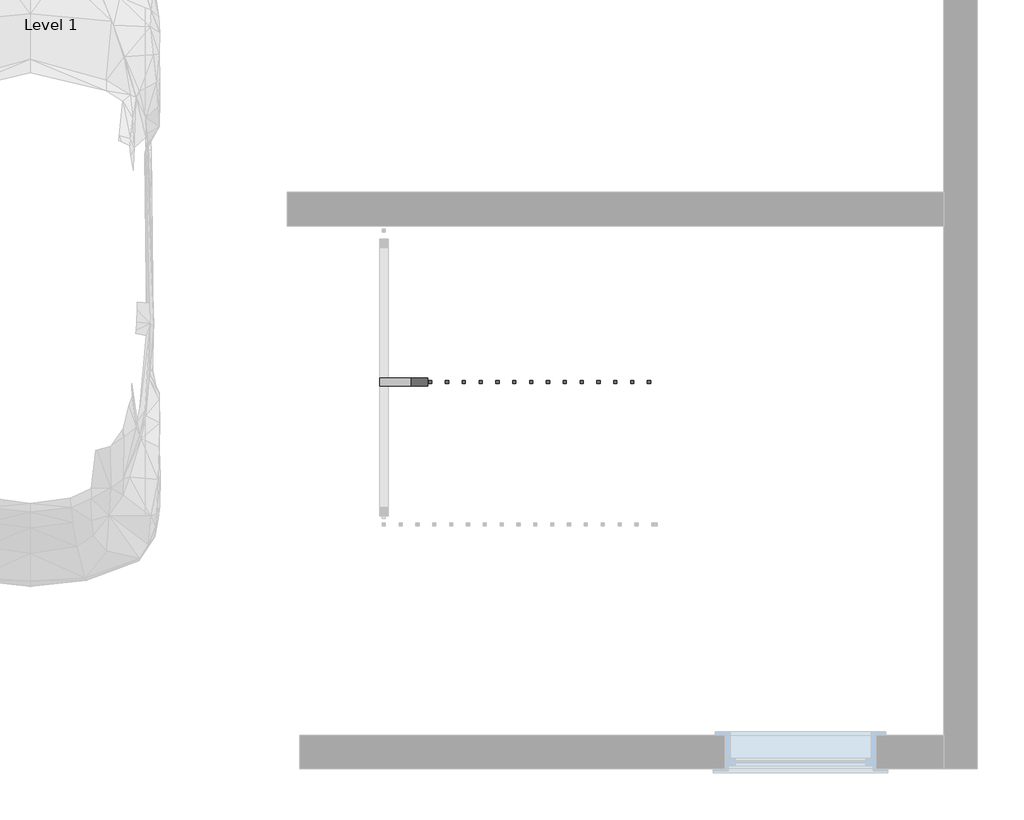
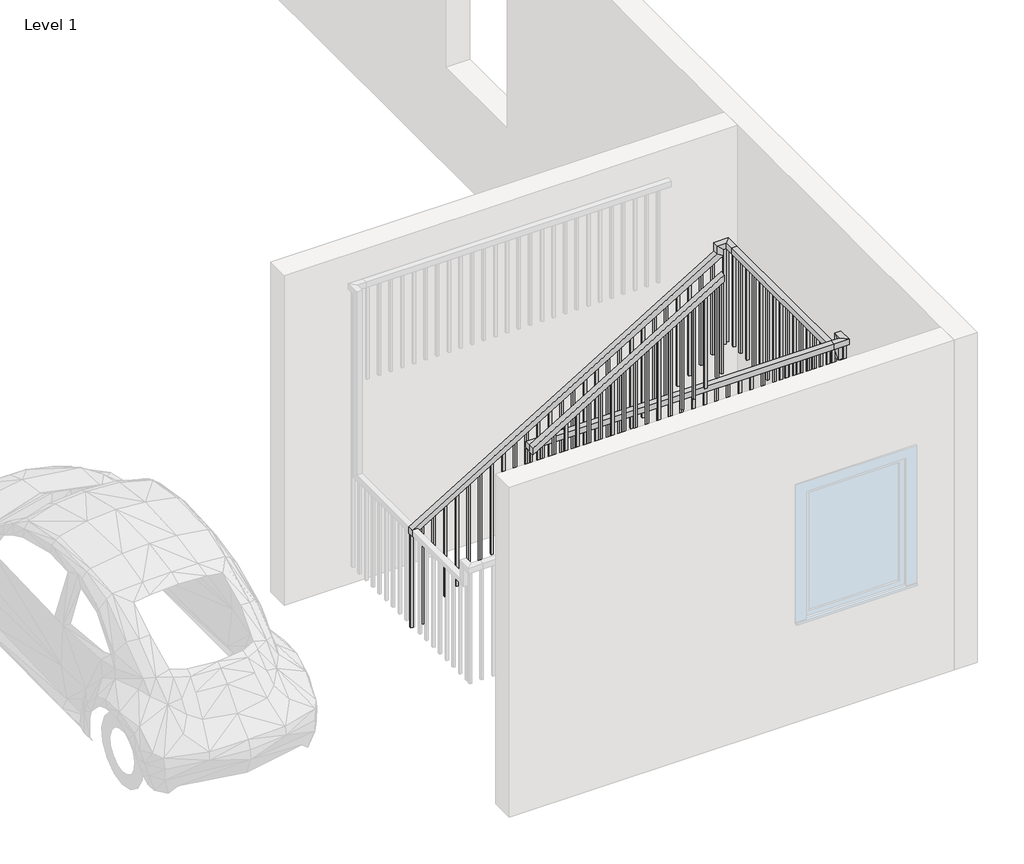
# One storey, part 2 of 3: 1 railing.
"""IFC4 building model written with IfcOpenShell, lengths in millimetres."""

from ifc_helpers import new_model, si_unit, frame, origin, place, context, project, spatial, polyline, outline, extrude, faceted_brep, element, save

model = new_model("IFC4")

# Units and contexts
model_context = context("Model", 3, world=origin())
ifc_project = project(units=[si_unit("LENGTHUNIT", "METRE", prefix="MILLI")], contexts=[model_context])

# Site, building, storey
site = spatial("IfcSite", under=ifc_project)
building = spatial("IfcBuilding", under=site)
storey = spatial("IfcBuildingStorey", under=building, Name="Level 1", Elevation=0.0)

# Railing
placement = place(None, origin())
element("IfcRailing", 1, ObjectType="Handrail - Rectangular", at=placement, inside=storey, context=model_context, shape_type="SolidModel", body=[
    faceted_brep([(-6389.1370113, -4999.3518521, 1083.7333333), (-6389.1370113, -4999.3518521, 1024.3318731), (-6389.1370113, -5050.1518521, 1024.3318731), (-6389.1370113, -5050.1518521, 1083.7333333), (-3722.1370113, -4999.3518521, 2700.0969697), (-3671.3370113, -4999.3518521, 2671.4833882), (-3671.3370113, -5050.1518521, 2671.4833882), (-3722.1370113, -5050.1518521, 2700.0969697), (-3722.1370113, -4999.3518521, 2777.0666667), (-3671.3370113, -4999.3518521, 2726.2666667), (-3671.3370113, -5050.1518521, 2726.2666667), (-3722.1370113, -5050.1518521, 2777.0666667), (-3595.1370113, -4999.3518521, 2777.0666667), (-3595.1370113, -4999.3518521, 2726.2666667), (-3645.9370113, -5050.1518521, 2726.2666667), (-3645.9370113, -5050.1518521, 2777.0666667), (-3595.1370113, -5126.3518521, 2777.0666667), (-3595.1370113, -5126.3518521, 2726.2666667), (-3645.9370113, -5126.3518521, 2726.2666667), (-3645.9370113, -5126.3518521, 2777.0666667), (-3595.1370113, -6697.0215145, 2777.0666667), (-3595.1370113, -6747.8215145, 2726.2666667), (-3645.9370113, -6747.8215145, 2726.2666667), (-3645.9370113, -6697.0215145, 2777.0666667), (-3595.1370113, -6697.0215145, 2946.4), (-3595.1370113, -6747.8215145, 2895.6), (-3645.9370113, -6747.8215145, 2895.6), (-3645.9370113, -6697.0215145, 2946.4), (-3595.1370113, -6824.0215145, 2946.4), (-3595.1370113, -6824.0215145, 2895.6), (-3645.9370113, -6773.2215145, 2895.6), (-3645.9370113, -6773.2215145, 2946.4), (-3722.1370113, -6824.0215145, 2946.4), (-3722.1370113, -6824.0215145, 2895.6), (-3722.1370113, -6773.2215145, 2895.6), (-3722.1370113, -6773.2215145, 2946.4), (-6389.1370113, -6824.0215145, 2946.4), (-6389.1370113, -6773.2215145, 2946.4), (-6389.1370113, -6773.2215145, 2895.6), (-6389.1370113, -6824.0215145, 2895.6)], [[[0, 1, 2, 3]], [[1, 0, 4, 5]], [[2, 1, 5, 6]], [[3, 2, 6, 7]], [[0, 3, 7, 4]], [[5, 4, 8, 9]], [[6, 5, 9, 10]], [[7, 6, 10, 11]], [[4, 7, 11, 8]], [[9, 8, 12, 13]], [[10, 9, 13, 14]], [[11, 10, 14, 15]], [[8, 11, 15, 12]], [[13, 12, 16, 17]], [[14, 13, 17, 18]], [[15, 14, 18, 19]], [[12, 15, 19, 16]], [[17, 16, 20, 21]], [[18, 17, 21, 22]], [[19, 18, 22, 23]], [[16, 19, 23, 20]], [[21, 20, 24, 25]], [[22, 21, 25, 26]], [[23, 22, 26, 27]], [[20, 23, 27, 24]], [[25, 24, 28, 29]], [[26, 25, 29, 30]], [[27, 26, 30, 31]], [[24, 27, 31, 28]], [[29, 28, 32, 33]], [[30, 29, 33, 34]], [[31, 30, 34, 35]], [[28, 31, 35, 32]], [[36, 37, 38, 39]], [[33, 32, 36, 39]], [[34, 33, 39, 38]], [[35, 34, 38, 37]], [[32, 35, 37, 36]]]),
    faceted_brep([(-6389.1370113, -6824.0215145, 2946.4), (-6389.1370113, -6824.0215145, 2886.9985397), (-6389.1370113, -6874.8215145, 2886.9985397), (-6389.1370113, -6874.8215145, 2946.4), (-4712.7370113, -6824.0215145, 3962.4), (-4712.7370113, -6874.8215145, 3962.4), (-4712.7370113, -6874.8215145, 3902.9985397), (-4712.7370113, -6824.0215145, 3902.9985397)], [[[0, 1, 2, 3]], [[4, 5, 6, 7]], [[1, 0, 4, 7]], [[2, 1, 7, 6]], [[3, 2, 6, 5]], [[0, 3, 5, 4]]]),
    extrude(outline(polyline([(3866.4379337, -4773.0620113), (3017.2121212, -4773.0620113), (3017.2121212, -4754.0120113), (3877.9833882, -4754.0120113), (3866.4379337, -4773.0620113)])), frame((0.0, -6858.9465145, 0.0), z_axis=(0.0, 1.0, 0.0), x_axis=(0.0, 0.0, 1.0)), (0.0, 0.0, 1.0), 19.05),
    extrude(outline(polyline([(3804.8621761, -4874.6620113), (2955.6363636, -4874.6620113), (2955.6363636, -4855.6120113), (3816.4076307, -4855.6120113), (3804.8621761, -4874.6620113)])), frame((0.0, -6858.9465145, 0.0), z_axis=(0.0, 1.0, 0.0), x_axis=(0.0, 0.0, 1.0)), (0.0, 0.0, 1.0), 19.05),
    extrude(outline(polyline([(3743.2864185, -4976.2620113), (2894.0606061, -4976.2620113), (2894.0606061, -4957.2120113), (3754.8318731, -4957.2120113), (3743.2864185, -4976.2620113)])), frame((0.0, -6858.9465145, 0.0), z_axis=(0.0, 1.0, 0.0), x_axis=(0.0, 0.0, 1.0)), (0.0, 0.0, 1.0), 19.05),
    extrude(outline(polyline([(3681.710661, -5077.8620113), (2832.4848485, -5077.8620113), (2832.4848485, -5058.8120113), (3693.2561155, -5058.8120113), (3681.710661, -5077.8620113)])), frame((0.0, -6858.9465145, 0.0), z_axis=(0.0, 1.0, 0.0), x_axis=(0.0, 0.0, 1.0)), (0.0, 0.0, 1.0), 19.05),
    extrude(outline(polyline([(3620.1349034, -5179.4620113), (2770.9090909, -5179.4620113), (2770.9090909, -5160.4120113), (3631.6803579, -5160.4120113), (3620.1349034, -5179.4620113)])), frame((0.0, -6858.9465145, 0.0), z_axis=(0.0, 1.0, 0.0), x_axis=(0.0, 0.0, 1.0)), (0.0, 0.0, 1.0), 19.05),
    extrude(outline(polyline([(3558.5591458, -5281.0620113), (2709.3333333, -5281.0620113), (2709.3333333, -5262.0120113), (3570.1046004, -5262.0120113), (3558.5591458, -5281.0620113)])), frame((0.0, -6858.9465145, 0.0), z_axis=(0.0, 1.0, 0.0), x_axis=(0.0, 0.0, 1.0)), (0.0, 0.0, 1.0), 19.05),
    extrude(outline(polyline([(3496.9833882, -5382.6620113), (2647.7575758, -5382.6620113), (2647.7575758, -5363.6120113), (3508.5288428, -5363.6120113), (3496.9833882, -5382.6620113)])), frame((0.0, -6858.9465145, 0.0), z_axis=(0.0, 1.0, 0.0), x_axis=(0.0, 0.0, 1.0)), (0.0, 0.0, 1.0), 19.05),
    extrude(outline(polyline([(3435.4076307, -5484.2620113), (2586.1818182, -5484.2620113), (2586.1818182, -5465.2120113), (3446.9530852, -5465.2120113), (3435.4076307, -5484.2620113)])), frame((0.0, -6858.9465145, 0.0), z_axis=(0.0, 1.0, 0.0), x_axis=(0.0, 0.0, 1.0)), (0.0, 0.0, 1.0), 19.05),
    extrude(outline(polyline([(3373.8318731, -5585.8620113), (2524.6060606, -5585.8620113), (2524.6060606, -5566.8120113), (3385.3773276, -5566.8120113), (3373.8318731, -5585.8620113)])), frame((0.0, -6858.9465145, 0.0), z_axis=(0.0, 1.0, 0.0), x_axis=(0.0, 0.0, 1.0)), (0.0, 0.0, 1.0), 19.05),
    extrude(outline(polyline([(3312.2561155, -5687.4620113), (2463.030303, -5687.4620113), (2463.030303, -5668.4120113), (3323.80157, -5668.4120113), (3312.2561155, -5687.4620113)])), frame((0.0, -6858.9465145, 0.0), z_axis=(0.0, 1.0, 0.0), x_axis=(0.0, 0.0, 1.0)), (0.0, 0.0, 1.0), 19.05),
    extrude(outline(polyline([(3250.6803579, -5789.0620113), (2401.4545455, -5789.0620113), (2401.4545455, -5770.0120113), (3262.2258125, -5770.0120113), (3250.6803579, -5789.0620113)])), frame((0.0, -6858.9465145, 0.0), z_axis=(0.0, 1.0, 0.0), x_axis=(0.0, 0.0, 1.0)), (0.0, 0.0, 1.0), 19.05),
    extrude(outline(polyline([(3189.1046004, -5890.6620113), (2339.8787879, -5890.6620113), (2339.8787879, -5871.6120113), (3200.6500549, -5871.6120113), (3189.1046004, -5890.6620113)])), frame((0.0, -6858.9465145, 0.0), z_axis=(0.0, 1.0, 0.0), x_axis=(0.0, 0.0, 1.0)), (0.0, 0.0, 1.0), 19.05),
    extrude(outline(polyline([(3127.5288428, -5992.2620113), (2278.3030303, -5992.2620113), (2278.3030303, -5973.2120113), (3139.0742973, -5973.2120113), (3127.5288428, -5992.2620113)])), frame((0.0, -6858.9465145, 0.0), z_axis=(0.0, 1.0, 0.0), x_axis=(0.0, 0.0, 1.0)), (0.0, 0.0, 1.0), 19.05),
    extrude(outline(polyline([(3065.9530852, -6093.8620113), (2108.2, -6093.8620113), (2108.2, -6074.8120113), (3077.4985397, -6074.8120113), (3065.9530852, -6093.8620113)])), frame((0.0, -6858.9465145, 0.0), z_axis=(0.0, 1.0, 0.0), x_axis=(0.0, 0.0, 1.0)), (0.0, 0.0, 1.0), 19.05),
    extrude(outline(polyline([(3004.3773276, -6195.4620113), (2108.2, -6195.4620113), (2108.2, -6176.4120113), (3015.9227822, -6176.4120113), (3004.3773276, -6195.4620113)])), frame((0.0, -6858.9465145, 0.0), z_axis=(0.0, 1.0, 0.0), x_axis=(0.0, 0.0, 1.0)), (0.0, 0.0, 1.0), 19.05),
    extrude(outline(polyline([(2942.80157, -6297.0620113), (2108.2, -6297.0620113), (2108.2, -6278.0120113), (2954.3470246, -6278.0120113), (2942.80157, -6297.0620113)])), frame((0.0, -6858.9465145, 0.0), z_axis=(0.0, 1.0, 0.0), x_axis=(0.0, 0.0, 1.0)), (0.0, 0.0, 1.0), 19.05),
    extrude(outline(polyline([(-6354.2120113, -6808.1465145), (-6373.2620113, -6808.1465145), (-6373.2620113, -6789.0965145), (-6354.2120113, -6789.0965145), (-6354.2120113, -6808.1465145)])), frame((0.0, 0.0, 2032.0), z_axis=(0.0, 0.0, 1.0), x_axis=(1.0, 0.0, 0.0)), (0.0, 0.0, 1.0), 863.6),
    extrude(outline(polyline([(2895.6, -6271.6620113), (2157.5236029, -6271.6620113), (2145.9781483, -6252.6120113), (2895.6, -6252.6120113), (2895.6, -6271.6620113)])), frame((0.0, -6808.1465145, 0.0), z_axis=(0.0, 1.0, 0.0), x_axis=(0.0, 0.0, 1.0)), (0.0, 0.0, 1.0), 19.05),
    extrude(outline(polyline([(2895.6, -6170.0620113), (2219.0993604, -6170.0620113), (2207.5539059, -6151.0120113), (2895.6, -6151.0120113), (2895.6, -6170.0620113)])), frame((0.0, -6808.1465145, 0.0), z_axis=(0.0, 1.0, 0.0), x_axis=(0.0, 0.0, 1.0)), (0.0, 0.0, 1.0), 19.05),
    extrude(outline(polyline([(2895.6, -6068.4620113), (2280.675118, -6068.4620113), (2269.1296635, -6049.4120113), (2895.6, -6049.4120113), (2895.6, -6068.4620113)])), frame((0.0, -6808.1465145, 0.0), z_axis=(0.0, 1.0, 0.0), x_axis=(0.0, 0.0, 1.0)), (0.0, 0.0, 1.0), 19.05),
    extrude(outline(polyline([(2895.6, -5966.8620113), (2342.2508756, -5966.8620113), (2330.7054211, -5947.8120113), (2895.6, -5947.8120113), (2895.6, -5966.8620113)])), frame((0.0, -6808.1465145, 0.0), z_axis=(0.0, 1.0, 0.0), x_axis=(0.0, 0.0, 1.0)), (0.0, 0.0, 1.0), 19.05),
    extrude(outline(polyline([(-5846.2120113, -6808.1465145), (-5865.2620113, -6808.1465145), (-5865.2620113, -6789.0965145), (-5846.2120113, -6789.0965145), (-5846.2120113, -6808.1465145)])), frame((0.0, 0.0, 2032.0), z_axis=(0.0, 0.0, 1.0), x_axis=(1.0, 0.0, 0.0)), (0.0, 0.0, 1.0), 863.6),
    extrude(outline(polyline([(-5744.6120113, -6808.1465145), (-5763.6620113, -6808.1465145), (-5763.6620113, -6789.0965145), (-5744.6120113, -6789.0965145), (-5744.6120113, -6808.1465145)])), frame((0.0, 0.0, 2032.0), z_axis=(0.0, 0.0, 1.0), x_axis=(1.0, 0.0, 0.0)), (0.0, 0.0, 1.0), 863.6),
    extrude(outline(polyline([(-5643.0120113, -6808.1465145), (-5662.0620113, -6808.1465145), (-5662.0620113, -6789.0965145), (-5643.0120113, -6789.0965145), (-5643.0120113, -6808.1465145)])), frame((0.0, 0.0, 2032.0), z_axis=(0.0, 0.0, 1.0), x_axis=(1.0, 0.0, 0.0)), (0.0, 0.0, 1.0), 863.6),
    extrude(outline(polyline([(-5541.4120113, -6808.1465145), (-5560.4620113, -6808.1465145), (-5560.4620113, -6789.0965145), (-5541.4120113, -6789.0965145), (-5541.4120113, -6808.1465145)])), frame((0.0, 0.0, 2032.0), z_axis=(0.0, 0.0, 1.0), x_axis=(1.0, 0.0, 0.0)), (0.0, 0.0, 1.0), 863.6),
    extrude(outline(polyline([(-5439.8120113, -6808.1465145), (-5458.8620113, -6808.1465145), (-5458.8620113, -6789.0965145), (-5439.8120113, -6789.0965145), (-5439.8120113, -6808.1465145)])), frame((0.0, 0.0, 2032.0), z_axis=(0.0, 0.0, 1.0), x_axis=(1.0, 0.0, 0.0)), (0.0, 0.0, 1.0), 863.6),
    extrude(outline(polyline([(-5338.2120113, -6808.1465145), (-5357.2620113, -6808.1465145), (-5357.2620113, -6789.0965145), (-5338.2120113, -6789.0965145), (-5338.2120113, -6808.1465145)])), frame((0.0, 0.0, 2032.0), z_axis=(0.0, 0.0, 1.0), x_axis=(1.0, 0.0, 0.0)), (0.0, 0.0, 1.0), 863.6),
    extrude(outline(polyline([(-5236.6120113, -6808.1465145), (-5255.6620113, -6808.1465145), (-5255.6620113, -6789.0965145), (-5236.6120113, -6789.0965145), (-5236.6120113, -6808.1465145)])), frame((0.0, 0.0, 2032.0), z_axis=(0.0, 0.0, 1.0), x_axis=(1.0, 0.0, 0.0)), (0.0, 0.0, 1.0), 863.6),
    extrude(outline(polyline([(-5135.0120113, -6808.1465145), (-5154.0620113, -6808.1465145), (-5154.0620113, -6789.0965145), (-5135.0120113, -6789.0965145), (-5135.0120113, -6808.1465145)])), frame((0.0, 0.0, 2032.0), z_axis=(0.0, 0.0, 1.0), x_axis=(1.0, 0.0, 0.0)), (0.0, 0.0, 1.0), 863.6),
    extrude(outline(polyline([(-5033.4120113, -6808.1465145), (-5052.4620113, -6808.1465145), (-5052.4620113, -6789.0965145), (-5033.4120113, -6789.0965145), (-5033.4120113, -6808.1465145)])), frame((0.0, 0.0, 2032.0), z_axis=(0.0, 0.0, 1.0), x_axis=(1.0, 0.0, 0.0)), (0.0, 0.0, 1.0), 863.6),
    extrude(outline(polyline([(-4931.8120113, -6808.1465145), (-4950.8620113, -6808.1465145), (-4950.8620113, -6789.0965145), (-4931.8120113, -6789.0965145), (-4931.8120113, -6808.1465145)])), frame((0.0, 0.0, 2032.0), z_axis=(0.0, 0.0, 1.0), x_axis=(1.0, 0.0, 0.0)), (0.0, 0.0, 1.0), 863.6),
    extrude(outline(polyline([(-4830.2120113, -6808.1465145), (-4849.2620113, -6808.1465145), (-4849.2620113, -6789.0965145), (-4830.2120113, -6789.0965145), (-4830.2120113, -6808.1465145)])), frame((0.0, 0.0, 2032.0), z_axis=(0.0, 0.0, 1.0), x_axis=(1.0, 0.0, 0.0)), (0.0, 0.0, 1.0), 863.6),
    extrude(outline(polyline([(-4728.6120113, -6808.1465145), (-4747.6620113, -6808.1465145), (-4747.6620113, -6789.0965145), (-4728.6120113, -6789.0965145), (-4728.6120113, -6808.1465145)])), frame((0.0, 0.0, 2032.0), z_axis=(0.0, 0.0, 1.0), x_axis=(1.0, 0.0, 0.0)), (0.0, 0.0, 1.0), 863.6),
    extrude(outline(polyline([(-4627.0120113, -6808.1465145), (-4646.0620113, -6808.1465145), (-4646.0620113, -6789.0965145), (-4627.0120113, -6789.0965145), (-4627.0120113, -6808.1465145)])), frame((0.0, 0.0, 2032.0), z_axis=(0.0, 0.0, 1.0), x_axis=(1.0, 0.0, 0.0)), (0.0, 0.0, 1.0), 863.6),
    extrude(outline(polyline([(-4525.4120113, -6808.1465145), (-4544.4620113, -6808.1465145), (-4544.4620113, -6789.0965145), (-4525.4120113, -6789.0965145), (-4525.4120113, -6808.1465145)])), frame((0.0, 0.0, 2032.0), z_axis=(0.0, 0.0, 1.0), x_axis=(1.0, 0.0, 0.0)), (0.0, 0.0, 1.0), 863.6),
    extrude(outline(polyline([(-4423.8120113, -6808.1465145), (-4442.8620113, -6808.1465145), (-4442.8620113, -6789.0965145), (-4423.8120113, -6789.0965145), (-4423.8120113, -6808.1465145)])), frame((0.0, 0.0, 2032.0), z_axis=(0.0, 0.0, 1.0), x_axis=(1.0, 0.0, 0.0)), (0.0, 0.0, 1.0), 863.6),
    extrude(outline(polyline([(-4322.2120113, -6808.1465145), (-4341.2620113, -6808.1465145), (-4341.2620113, -6789.0965145), (-4322.2120113, -6789.0965145), (-4322.2120113, -6808.1465145)])), frame((0.0, 0.0, 2032.0), z_axis=(0.0, 0.0, 1.0), x_axis=(1.0, 0.0, 0.0)), (0.0, 0.0, 1.0), 863.6),
    extrude(outline(polyline([(-4220.6120113, -6808.1465145), (-4239.6620113, -6808.1465145), (-4239.6620113, -6789.0965145), (-4220.6120113, -6789.0965145), (-4220.6120113, -6808.1465145)])), frame((0.0, 0.0, 2032.0), z_axis=(0.0, 0.0, 1.0), x_axis=(1.0, 0.0, 0.0)), (0.0, 0.0, 1.0), 863.6),
    extrude(outline(polyline([(-4119.0120113, -6808.1465145), (-4138.0620113, -6808.1465145), (-4138.0620113, -6789.0965145), (-4119.0120113, -6789.0965145), (-4119.0120113, -6808.1465145)])), frame((0.0, 0.0, 2032.0), z_axis=(0.0, 0.0, 1.0), x_axis=(1.0, 0.0, 0.0)), (0.0, 0.0, 1.0), 863.6),
    extrude(outline(polyline([(-4017.4120113, -6808.1465145), (-4036.4620113, -6808.1465145), (-4036.4620113, -6789.0965145), (-4017.4120113, -6789.0965145), (-4017.4120113, -6808.1465145)])), frame((0.0, 0.0, 2032.0), z_axis=(0.0, 0.0, 1.0), x_axis=(1.0, 0.0, 0.0)), (0.0, 0.0, 1.0), 863.6),
    extrude(outline(polyline([(-3915.8120113, -6808.1465145), (-3934.8620113, -6808.1465145), (-3934.8620113, -6789.0965145), (-3915.8120113, -6789.0965145), (-3915.8120113, -6808.1465145)])), frame((0.0, 0.0, 2032.0), z_axis=(0.0, 0.0, 1.0), x_axis=(1.0, 0.0, 0.0)), (0.0, 0.0, 1.0), 863.6),
    extrude(outline(polyline([(-3814.2120113, -6808.1465145), (-3833.2620113, -6808.1465145), (-3833.2620113, -6789.0965145), (-3814.2120113, -6789.0965145), (-3814.2120113, -6808.1465145)])), frame((0.0, 0.0, 2032.0), z_axis=(0.0, 0.0, 1.0), x_axis=(1.0, 0.0, 0.0)), (0.0, 0.0, 1.0), 863.6),
    extrude(outline(polyline([(-3712.6120113, -6808.1465145), (-3731.6620113, -6808.1465145), (-3731.6620113, -6789.0965145), (-3712.6120113, -6789.0965145), (-3712.6120113, -6808.1465145)])), frame((0.0, 0.0, 2032.0), z_axis=(0.0, 0.0, 1.0), x_axis=(1.0, 0.0, 0.0)), (0.0, 0.0, 1.0), 863.6),
    extrude(outline(polyline([(-3611.0120113, -6742.4268521), (-3611.0120113, -6761.4768521), (-3630.0620113, -6761.4768521), (-3630.0620113, -6742.4268521), (-3611.0120113, -6742.4268521)])), frame((0.0, 0.0, 1862.6666667), z_axis=(0.0, 0.0, 1.0), x_axis=(1.0, 0.0, 0.0)), (0.0, 0.0, 1.0), 863.6),
    extrude(outline(polyline([(-3611.0120113, -6640.8268521), (-3611.0120113, -6659.8768521), (-3630.0620113, -6659.8768521), (-3630.0620113, -6640.8268521), (-3611.0120113, -6640.8268521)])), frame((0.0, 0.0, 1862.6666667), z_axis=(0.0, 0.0, 1.0), x_axis=(1.0, 0.0, 0.0)), (0.0, 0.0, 1.0), 863.6),
    extrude(outline(polyline([(-3611.0120113, -6539.2268521), (-3611.0120113, -6558.2768521), (-3630.0620113, -6558.2768521), (-3630.0620113, -6539.2268521), (-3611.0120113, -6539.2268521)])), frame((0.0, 0.0, 1862.6666667), z_axis=(0.0, 0.0, 1.0), x_axis=(1.0, 0.0, 0.0)), (0.0, 0.0, 1.0), 863.6),
    extrude(outline(polyline([(-3611.0120113, -6437.6268521), (-3611.0120113, -6456.6768521), (-3630.0620113, -6456.6768521), (-3630.0620113, -6437.6268521), (-3611.0120113, -6437.6268521)])), frame((0.0, 0.0, 1862.6666667), z_axis=(0.0, 0.0, 1.0), x_axis=(1.0, 0.0, 0.0)), (0.0, 0.0, 1.0), 863.6),
    extrude(outline(polyline([(-3611.0120113, -6336.0268521), (-3611.0120113, -6355.0768521), (-3630.0620113, -6355.0768521), (-3630.0620113, -6336.0268521), (-3611.0120113, -6336.0268521)])), frame((0.0, 0.0, 1862.6666667), z_axis=(0.0, 0.0, 1.0), x_axis=(1.0, 0.0, 0.0)), (0.0, 0.0, 1.0), 863.6),
    extrude(outline(polyline([(-3611.0120113, -6234.4268521), (-3611.0120113, -6253.4768521), (-3630.0620113, -6253.4768521), (-3630.0620113, -6234.4268521), (-3611.0120113, -6234.4268521)])), frame((0.0, 0.0, 1862.6666667), z_axis=(0.0, 0.0, 1.0), x_axis=(1.0, 0.0, 0.0)), (0.0, 0.0, 1.0), 863.6),
    extrude(outline(polyline([(-3611.0120113, -6132.8268521), (-3611.0120113, -6151.8768521), (-3630.0620113, -6151.8768521), (-3630.0620113, -6132.8268521), (-3611.0120113, -6132.8268521)])), frame((0.0, 0.0, 1862.6666667), z_axis=(0.0, 0.0, 1.0), x_axis=(1.0, 0.0, 0.0)), (0.0, 0.0, 1.0), 863.6),
    extrude(outline(polyline([(-3611.0120113, -6031.2268521), (-3611.0120113, -6050.2768521), (-3630.0620113, -6050.2768521), (-3630.0620113, -6031.2268521), (-3611.0120113, -6031.2268521)])), frame((0.0, 0.0, 1862.6666667), z_axis=(0.0, 0.0, 1.0), x_axis=(1.0, 0.0, 0.0)), (0.0, 0.0, 1.0), 863.6),
    extrude(outline(polyline([(-3611.0120113, -5929.6268521), (-3611.0120113, -5948.6768521), (-3630.0620113, -5948.6768521), (-3630.0620113, -5929.6268521), (-3611.0120113, -5929.6268521)])), frame((0.0, 0.0, 1862.6666667), z_axis=(0.0, 0.0, 1.0), x_axis=(1.0, 0.0, 0.0)), (0.0, 0.0, 1.0), 863.6),
    extrude(outline(polyline([(-3611.0120113, -5828.0268521), (-3611.0120113, -5847.0768521), (-3630.0620113, -5847.0768521), (-3630.0620113, -5828.0268521), (-3611.0120113, -5828.0268521)])), frame((0.0, 0.0, 1862.6666667), z_axis=(0.0, 0.0, 1.0), x_axis=(1.0, 0.0, 0.0)), (0.0, 0.0, 1.0), 863.6),
    extrude(outline(polyline([(-3611.0120113, -5726.4268521), (-3611.0120113, -5745.4768521), (-3630.0620113, -5745.4768521), (-3630.0620113, -5726.4268521), (-3611.0120113, -5726.4268521)])), frame((0.0, 0.0, 1862.6666667), z_axis=(0.0, 0.0, 1.0), x_axis=(1.0, 0.0, 0.0)), (0.0, 0.0, 1.0), 863.6),
    extrude(outline(polyline([(-3611.0120113, -5624.8268521), (-3611.0120113, -5643.8768521), (-3630.0620113, -5643.8768521), (-3630.0620113, -5624.8268521), (-3611.0120113, -5624.8268521)])), frame((0.0, 0.0, 1862.6666667), z_axis=(0.0, 0.0, 1.0), x_axis=(1.0, 0.0, 0.0)), (0.0, 0.0, 1.0), 863.6),
    extrude(outline(polyline([(-3611.0120113, -5523.2268521), (-3611.0120113, -5542.2768521), (-3630.0620113, -5542.2768521), (-3630.0620113, -5523.2268521), (-3611.0120113, -5523.2268521)])), frame((0.0, 0.0, 1862.6666667), z_axis=(0.0, 0.0, 1.0), x_axis=(1.0, 0.0, 0.0)), (0.0, 0.0, 1.0), 863.6),
    extrude(outline(polyline([(-3611.0120113, -5421.6268521), (-3611.0120113, -5440.6768521), (-3630.0620113, -5440.6768521), (-3630.0620113, -5421.6268521), (-3611.0120113, -5421.6268521)])), frame((0.0, 0.0, 1862.6666667), z_axis=(0.0, 0.0, 1.0), x_axis=(1.0, 0.0, 0.0)), (0.0, 0.0, 1.0), 863.6),
    extrude(outline(polyline([(-3611.0120113, -5320.0268521), (-3611.0120113, -5339.0768521), (-3630.0620113, -5339.0768521), (-3630.0620113, -5320.0268521), (-3611.0120113, -5320.0268521)])), frame((0.0, 0.0, 1862.6666667), z_axis=(0.0, 0.0, 1.0), x_axis=(1.0, 0.0, 0.0)), (0.0, 0.0, 1.0), 863.6),
    extrude(outline(polyline([(-3611.0120113, -5218.4268521), (-3611.0120113, -5237.4768521), (-3630.0620113, -5237.4768521), (-3630.0620113, -5218.4268521), (-3611.0120113, -5218.4268521)])), frame((0.0, 0.0, 1862.6666667), z_axis=(0.0, 0.0, 1.0), x_axis=(1.0, 0.0, 0.0)), (0.0, 0.0, 1.0), 863.6),
    extrude(outline(polyline([(-3611.0120113, -5116.8268521), (-3611.0120113, -5135.8768521), (-3630.0620113, -5135.8768521), (-3630.0620113, -5116.8268521), (-3611.0120113, -5116.8268521)])), frame((0.0, 0.0, 1862.6666667), z_axis=(0.0, 0.0, 1.0), x_axis=(1.0, 0.0, 0.0)), (0.0, 0.0, 1.0), 863.6),
    extrude(outline(polyline([(-3655.4620113, -5015.2268521), (-3636.4120113, -5015.2268521), (-3636.4120113, -5034.2768521), (-3655.4620113, -5034.2768521), (-3655.4620113, -5015.2268521)])), frame((0.0, 0.0, 1831.8787879), z_axis=(0.0, 0.0, 1.0), x_axis=(1.0, 0.0, 0.0)), (0.0, 0.0, 1.0), 894.3878788),
    extrude(outline(polyline([(2619.5288428, -3757.0620113), (1770.3030303, -3757.0620113), (1770.3030303, -3738.0120113), (2631.0742973, -3738.0120113), (2619.5288428, -3757.0620113)])), frame((0.0, -5034.2768521, 0.0), z_axis=(0.0, 1.0, 0.0), x_axis=(0.0, 0.0, 1.0)), (0.0, 0.0, 1.0), 19.05),
    extrude(outline(polyline([(2557.9530852, -3858.6620113), (1708.7272727, -3858.6620113), (1708.7272727, -3839.6120113), (2569.4985397, -3839.6120113), (2557.9530852, -3858.6620113)])), frame((0.0, -5034.2768521, 0.0), z_axis=(0.0, 1.0, 0.0), x_axis=(0.0, 0.0, 1.0)), (0.0, 0.0, 1.0), 19.05),
    extrude(outline(polyline([(2496.3773276, -3960.2620113), (1647.1515152, -3960.2620113), (1647.1515152, -3941.2120113), (2507.9227822, -3941.2120113), (2496.3773276, -3960.2620113)])), frame((0.0, -5034.2768521, 0.0), z_axis=(0.0, 1.0, 0.0), x_axis=(0.0, 0.0, 1.0)), (0.0, 0.0, 1.0), 19.05),
    extrude(outline(polyline([(2434.80157, -4061.8620113), (1585.5757576, -4061.8620113), (1585.5757576, -4042.8120113), (2446.3470246, -4042.8120113), (2434.80157, -4061.8620113)])), frame((0.0, -5034.2768521, 0.0), z_axis=(0.0, 1.0, 0.0), x_axis=(0.0, 0.0, 1.0)), (0.0, 0.0, 1.0), 19.05),
    extrude(outline(polyline([(2373.2258125, -4163.4620113), (1524.0, -4163.4620113), (1524.0, -4144.4120113), (2384.771267, -4144.4120113), (2373.2258125, -4163.4620113)])), frame((0.0, -5034.2768521, 0.0), z_axis=(0.0, 1.0, 0.0), x_axis=(0.0, 0.0, 1.0)), (0.0, 0.0, 1.0), 19.05),
    extrude(outline(polyline([(2311.6500549, -4265.0620113), (1462.4242424, -4265.0620113), (1462.4242424, -4246.0120113), (2323.1955094, -4246.0120113), (2311.6500549, -4265.0620113)])), frame((0.0, -5034.2768521, 0.0), z_axis=(0.0, 1.0, 0.0), x_axis=(0.0, 0.0, 1.0)), (0.0, 0.0, 1.0), 19.05),
    extrude(outline(polyline([(2250.0742973, -4366.6620113), (1400.8484848, -4366.6620113), (1400.8484848, -4347.6120113), (2261.6197519, -4347.6120113), (2250.0742973, -4366.6620113)])), frame((0.0, -5034.2768521, 0.0), z_axis=(0.0, 1.0, 0.0), x_axis=(0.0, 0.0, 1.0)), (0.0, 0.0, 1.0), 19.05),
    extrude(outline(polyline([(2188.4985397, -4468.2620113), (1339.2727273, -4468.2620113), (1339.2727273, -4449.2120113), (2200.0439943, -4449.2120113), (2188.4985397, -4468.2620113)])), frame((0.0, -5034.2768521, 0.0), z_axis=(0.0, 1.0, 0.0), x_axis=(0.0, 0.0, 1.0)), (0.0, 0.0, 1.0), 19.05),
    extrude(outline(polyline([(2126.9227822, -4569.8620113), (1277.6969697, -4569.8620113), (1277.6969697, -4550.8120113), (2138.4682367, -4550.8120113), (2126.9227822, -4569.8620113)])), frame((0.0, -5034.2768521, 0.0), z_axis=(0.0, 1.0, 0.0), x_axis=(0.0, 0.0, 1.0)), (0.0, 0.0, 1.0), 19.05),
    extrude(outline(polyline([(2065.3470246, -4671.4620113), (1216.1212121, -4671.4620113), (1216.1212121, -4652.4120113), (2076.8924791, -4652.4120113), (2065.3470246, -4671.4620113)])), frame((0.0, -5034.2768521, 0.0), z_axis=(0.0, 1.0, 0.0), x_axis=(0.0, 0.0, 1.0)), (0.0, 0.0, 1.0), 19.05),
    extrude(outline(polyline([(2003.771267, -4773.0620113), (1154.5454545, -4773.0620113), (1154.5454545, -4754.0120113), (2015.3167216, -4754.0120113), (2003.771267, -4773.0620113)])), frame((0.0, -5034.2768521, 0.0), z_axis=(0.0, 1.0, 0.0), x_axis=(0.0, 0.0, 1.0)), (0.0, 0.0, 1.0), 19.05),
    extrude(outline(polyline([(1942.1955094, -4874.6620113), (1092.969697, -4874.6620113), (1092.969697, -4855.6120113), (1953.740964, -4855.6120113), (1942.1955094, -4874.6620113)])), frame((0.0, -5034.2768521, 0.0), z_axis=(0.0, 1.0, 0.0), x_axis=(0.0, 0.0, 1.0)), (0.0, 0.0, 1.0), 19.05),
    extrude(outline(polyline([(1880.6197519, -4976.2620113), (1031.3939394, -4976.2620113), (1031.3939394, -4957.2120113), (1892.1652064, -4957.2120113), (1880.6197519, -4976.2620113)])), frame((0.0, -5034.2768521, 0.0), z_axis=(0.0, 1.0, 0.0), x_axis=(0.0, 0.0, 1.0)), (0.0, 0.0, 1.0), 19.05),
    extrude(outline(polyline([(1819.0439943, -5077.8620113), (969.8181818, -5077.8620113), (969.8181818, -5058.8120113), (1830.5894488, -5058.8120113), (1819.0439943, -5077.8620113)])), frame((0.0, -5034.2768521, 0.0), z_axis=(0.0, 1.0, 0.0), x_axis=(0.0, 0.0, 1.0)), (0.0, 0.0, 1.0), 19.05),
    extrude(outline(polyline([(1757.4682367, -5179.4620113), (908.2424242, -5179.4620113), (908.2424242, -5160.4120113), (1769.0136913, -5160.4120113), (1757.4682367, -5179.4620113)])), frame((0.0, -5034.2768521, 0.0), z_axis=(0.0, 1.0, 0.0), x_axis=(0.0, 0.0, 1.0)), (0.0, 0.0, 1.0), 19.05),
    extrude(outline(polyline([(1695.8924791, -5281.0620113), (846.6666667, -5281.0620113), (846.6666667, -5262.0120113), (1707.4379337, -5262.0120113), (1695.8924791, -5281.0620113)])), frame((0.0, -5034.2768521, 0.0), z_axis=(0.0, 1.0, 0.0), x_axis=(0.0, 0.0, 1.0)), (0.0, 0.0, 1.0), 19.05),
    extrude(outline(polyline([(1634.3167216, -5382.6620113), (785.0909091, -5382.6620113), (785.0909091, -5363.6120113), (1645.8621761, -5363.6120113), (1634.3167216, -5382.6620113)])), frame((0.0, -5034.2768521, 0.0), z_axis=(0.0, 1.0, 0.0), x_axis=(0.0, 0.0, 1.0)), (0.0, 0.0, 1.0), 19.05),
    extrude(outline(polyline([(1572.740964, -5484.2620113), (723.5151515, -5484.2620113), (723.5151515, -5465.2120113), (1584.2864185, -5465.2120113), (1572.740964, -5484.2620113)])), frame((0.0, -5034.2768521, 0.0), z_axis=(0.0, 1.0, 0.0), x_axis=(0.0, 0.0, 1.0)), (0.0, 0.0, 1.0), 19.05),
    extrude(outline(polyline([(1511.1652064, -5585.8620113), (661.9393939, -5585.8620113), (661.9393939, -5566.8120113), (1522.710661, -5566.8120113), (1511.1652064, -5585.8620113)])), frame((0.0, -5034.2768521, 0.0), z_axis=(0.0, 1.0, 0.0), x_axis=(0.0, 0.0, 1.0)), (0.0, 0.0, 1.0), 19.05),
    extrude(outline(polyline([(1449.5894488, -5687.4620113), (600.3636364, -5687.4620113), (600.3636364, -5668.4120113), (1461.1349034, -5668.4120113), (1449.5894488, -5687.4620113)])), frame((0.0, -5034.2768521, 0.0), z_axis=(0.0, 1.0, 0.0), x_axis=(0.0, 0.0, 1.0)), (0.0, 0.0, 1.0), 19.05),
    extrude(outline(polyline([(1388.0136913, -5789.0620113), (538.7878788, -5789.0620113), (538.7878788, -5770.0120113), (1399.5591458, -5770.0120113), (1388.0136913, -5789.0620113)])), frame((0.0, -5034.2768521, 0.0), z_axis=(0.0, 1.0, 0.0), x_axis=(0.0, 0.0, 1.0)), (0.0, 0.0, 1.0), 19.05),
    extrude(outline(polyline([(1326.4379337, -5890.6620113), (477.2121212, -5890.6620113), (477.2121212, -5871.6120113), (1337.9833882, -5871.6120113), (1326.4379337, -5890.6620113)])), frame((0.0, -5034.2768521, 0.0), z_axis=(0.0, 1.0, 0.0), x_axis=(0.0, 0.0, 1.0)), (0.0, 0.0, 1.0), 19.05),
    extrude(outline(polyline([(1264.8621761, -5992.2620113), (415.6363636, -5992.2620113), (415.6363636, -5973.2120113), (1276.4076307, -5973.2120113), (1264.8621761, -5992.2620113)])), frame((0.0, -5034.2768521, 0.0), z_axis=(0.0, 1.0, 0.0), x_axis=(0.0, 0.0, 1.0)), (0.0, 0.0, 1.0), 19.05),
    extrude(outline(polyline([(1203.2864185, -6093.8620113), (354.0606061, -6093.8620113), (354.0606061, -6074.8120113), (1214.8318731, -6074.8120113), (1203.2864185, -6093.8620113)])), frame((0.0, -5034.2768521, 0.0), z_axis=(0.0, 1.0, 0.0), x_axis=(0.0, 0.0, 1.0)), (0.0, 0.0, 1.0), 19.05),
    extrude(outline(polyline([(1141.710661, -6195.4620113), (169.3333333, -6195.4620113), (169.3333333, -6176.4120113), (1153.2561155, -6176.4120113), (1141.710661, -6195.4620113)])), frame((0.0, -5034.2768521, 0.0), z_axis=(0.0, 1.0, 0.0), x_axis=(0.0, 0.0, 1.0)), (0.0, 0.0, 1.0), 19.05),
    extrude(outline(polyline([(1080.1349034, -6297.0620113), (169.3333333, -6297.0620113), (169.3333333, -6278.0120113), (1091.6803579, -6278.0120113), (1080.1349034, -6297.0620113)])), frame((0.0, -5034.2768521, 0.0), z_axis=(0.0, 1.0, 0.0), x_axis=(0.0, 0.0, 1.0)), (0.0, 0.0, 1.0), 19.05),
    extrude(outline(polyline([(-6379.6120113, -6808.1465145), (-6398.6620113, -6808.1465145), (-6398.6620113, -6789.0965145), (-6379.6120113, -6789.0965145), (-6379.6120113, -6808.1465145)])), frame((0.0, 0.0, 2032.0), z_axis=(0.0, 0.0, 1.0), x_axis=(1.0, 0.0, 0.0)), (0.0, 0.0, 1.0), 863.6),
    extrude(outline(polyline([(-3611.0120113, -6808.1465145), (-3630.0620113, -6808.1465145), (-3630.0620113, -6789.0965145), (-3611.0120113, -6789.0965145), (-3611.0120113, -6808.1465145)])), frame((0.0, 0.0, 1862.6666667), z_axis=(0.0, 0.0, 1.0), x_axis=(1.0, 0.0, 0.0)), (0.0, 0.0, 1.0), 1032.9333333),
    extrude(outline(polyline([(-3611.0120113, -5015.2268521), (-3611.0120113, -5034.2768521), (-3630.0620113, -5034.2768521), (-3630.0620113, -5015.2268521), (-3611.0120113, -5015.2268521)])), frame((0.0, 0.0, 1847.2727273), z_axis=(0.0, 0.0, 1.0), x_axis=(1.0, 0.0, 0.0)), (0.0, 0.0, 1.0), 878.9939394),
    extrude(outline(polyline([(3891.4530852, -4731.7870113), (3042.2272727, -4731.7870113), (3042.2272727, -4712.7370113), (3902.9985397, -4712.7370113), (3891.4530852, -4731.7870113)])), frame((0.0, -6858.9465145, 0.0), z_axis=(0.0, 1.0, 0.0), x_axis=(0.0, 0.0, 1.0)), (0.0, 0.0, 1.0), 19.05),
    extrude(outline(polyline([(1024.3318731, -6389.1370113), (169.3333333, -6389.1370113), (169.3333333, -6370.0870113), (1035.8773276, -6370.0870113), (1024.3318731, -6389.1370113)])), frame((0.0, -5034.2768521, 0.0), z_axis=(0.0, 1.0, 0.0), x_axis=(0.0, 0.0, 1.0)), (0.0, 0.0, 1.0), 19.05),
])

save(model, "model.ifc")

# Revit data of these elements
# Type "Handrail - Rectangular"
#   Assembly Code = "C2010400"
#   built-in parameter 1008612 = 0.0416667 (stored number, unit not read)
#   built-in parameter 1008611 = 0.0416667 (stored number, unit not read)
#   built-in parameter 1008609 = 0.333333 (stored number, unit not read)
#   built-in parameter 1008604 = 0.166667 (stored number, unit not read)
#   built-in parameter 1008603 = 0.166667 (stored number, unit not read)
#   Railing Height = 3' - 0"
#   built-in parameter 1008630 = 2
#   built-in parameter 1008610 = 2
#   built-in parameter 1008618 = Baluster - Square : 3/4"
# Element 1 (IfcRailing, "Handrail - Rectangular")
#   Phase Created = New Construction
